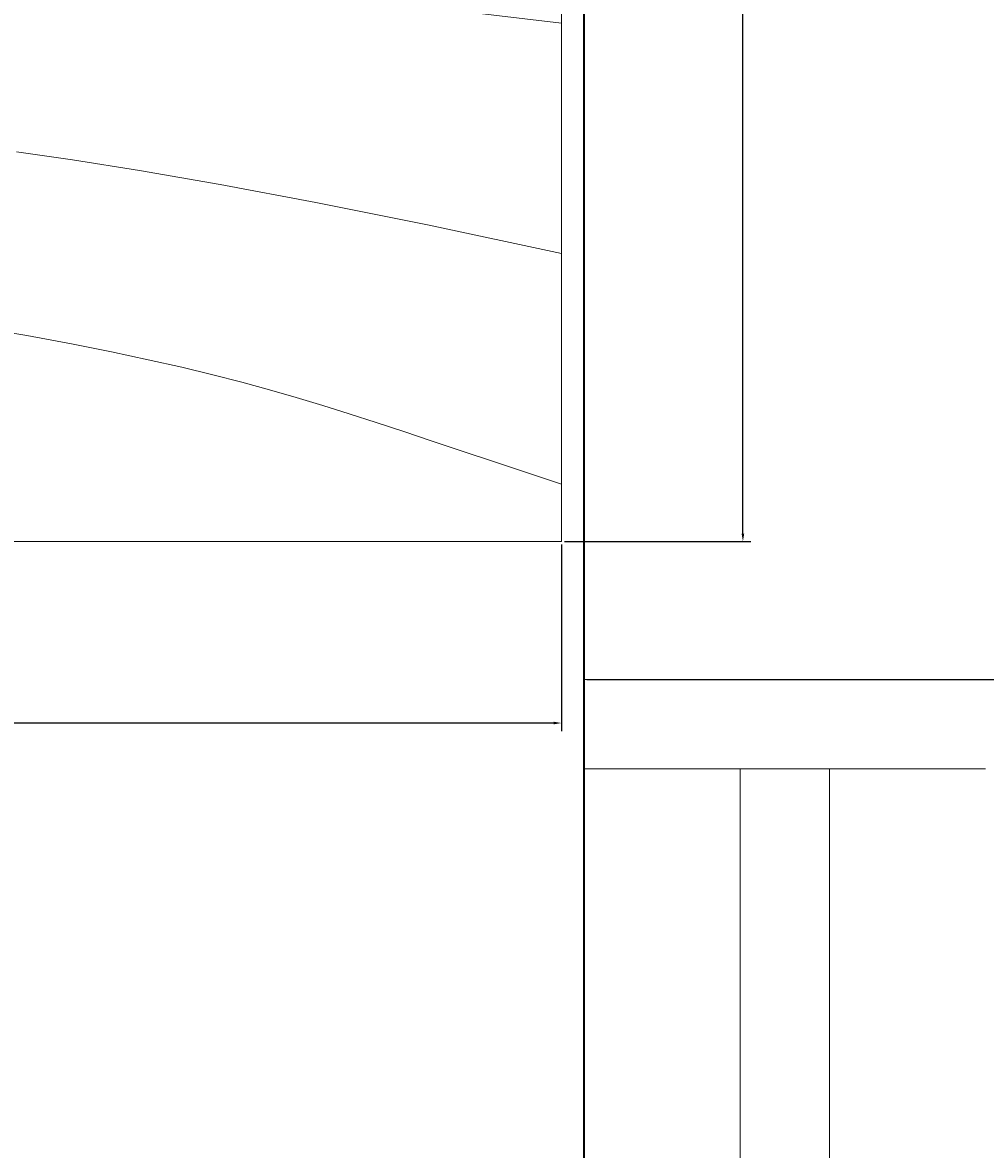
# Model space of a CAD drawing. Units: inches. Extents: x -128 to 854, y -395 to 398.
# Tile 39 of 61: x 292 to 314, y 145 to 170. Entities that reach past the tile are written whole.
import ezdxf

# ---------------------------------------------------------------- set-up
doc = ezdxf.new("R2010")
doc.units = ezdxf.units.IN
doc.header["$MEASUREMENT"] = 0
for name, color, linetype, lineweight in [('A-ANNO-DIMS', 2, 'Continuous', 18), ('A-FURN', 8, 'Continuous', 18), ('A-GLAZ', 220, 'Continuous', 18), ('A-WALL', 4, 'Continuous', 35)]:
    doc.layers.add(name, color=color, linetype=linetype, lineweight=lineweight)
doc.styles.get("Standard").update_dxf_attribs({"font": 'arial.ttf'})
doc.dimstyles.get("Standard").update_dxf_attribs({"dimtxt": 0.18, "dimasz": 0.18, "dimexe": 0.18, "dimexo": 0.0625, "dimgap": 0.09, "dimtad": 0, "dimtih": 1, "dimtoh": 1, "dimdec": 1, "dimzin": 0, "dimdsep": 46, "dimlunit": 4, "dimtxsty": 'Standard', "dimcen": 0.09, "dimclrd": 1, "dimclre": 2, "dimclrt": 6, "dimadec": 0, "dimazin": 0, "dimtfac": 1, "dimtdec": 1, "dimtofl": 0, "dimtmove": 0, "dimatfit": 3, "dimfxl": 1, "dimtfill": 2, "dimtfillclr": 3, "dimtolj": 1, "dimtzin": 0, "dimarcsym": 0})

# ---------------------------------------------------------------- blocks, each defined once
blk = doc.blocks.new('Table - Square Woodgrain 42 x 42 in.')
blk.add_line((0, -42), (42, -42))
for points in [[(0, -42), (0, 0), (42, 0), (42, -42)], [(0, -24), (3.9243, -23.6805), (7.4766, -23.4138), (10.6891, -23.1954), (13.5943, -23.0205), (16.2247, -22.8847), (18.6125, -22.7832), (20.7903, -22.7116), (22.7903, -22.6651), (24.6563, -22.642), (26.4764, -22.6507), (28.35, -22.7024), (30.3766, -22.8084), (32.6555, -22.98), (35.2861, -23.2283), (38.3678, -23.5645), (42, -24)], [(42, -32), (37.392, -31.017), (33.4585, -30.2231), (30.1291, -29.5949), (27.3334, -29.109), (25.0009, -28.742), (23.0612, -28.4707)], [(21.6171, -34.5413), (23.4136, -34.8486), (24.9657, -35.1382), (26.3614, -35.4156), (27.6332, -35.6841), (28.7995, -35.9467), (29.8788, -36.2064), (30.8897, -36.4661), (31.8507, -36.7288), (32.7802, -36.9973), (33.6968, -37.2747), (34.6175, -37.5635), (35.5531, -37.8651), (36.5128, -38.1805), (37.506, -38.5108), (38.5421, -38.8568), (39.6302, -39.2197), (40.7797, -39.6004), (42, -40)]]:
    blk.add_lwpolyline(points)
blk = doc.blocks.new('*D55')
at = {"layer": 'A-ANNO-DIMS', "color": 0, "lineweight": -2, "transparency": 16777216}
for p, q in [((304.81, 186.741), (221.092, 186.741)), ((221.272, 181.741), (221.272, 131.873)), ((221.272, 77.741), (221.272, 127.608)), ((304.81, 72.741), (221.092, 72.741))]:
    blk.add_line(p, q, dxfattribs=at)
at = {"layer": 'A-ANNO-DIMS', "color": 0, "transparency": 16777216}
for points in [[(220.439, 181.741), (222.105, 181.741), (221.272, 186.741)], [(220.439, 77.741), (222.105, 77.741), (221.272, 72.741)]]:
    blk.add_solid(points, dxfattribs=at)
at = {"layer": 'Defpoints', "color": 0, "transparency": 16777216}
for p in [(221.272, 186.741), (304.873, 186.741), (304.873, 72.741)]:
    blk.add_point(p, dxfattribs=at)
at = {"layer": 'A-ANNO-DIMS', "color": 0, "transparency": 16777216, "insert": (221.272, 129.741), "char_height": 4, "attachment_point": 5, "bg_fill": 1, "box_fill_scale": 1.25, "bg_fill_color": 3, "bg_fill_transparency": 0}
blk.add_mtext('\\A1;9\'-6"', dxfattribs=at)
blk = doc.blocks.new('WIN-48IN')
for p, q in [((9, 52), (0, 52)), ((9, 50), (0, 50)), ((3.5, 50), (3.5, 2)), ((5.5, 50), (5.5, 2))]:
    blk.add_line(p, q)
blk = doc.blocks.new('*D87')
at = {"layer": 'A-ANNO-DIMS', "color": 2, "lineweight": -2, "transparency": 16777216}
for p, q in [((304.435, 185.918), (308.616, 185.918)), ((304.435, 158.828), (308.616, 158.828))]:
    blk.add_line(p, q, dxfattribs=at)
at = {"layer": 'A-ANNO-DIMS', "color": 1, "lineweight": -2, "transparency": 16777216}
for p, q in [((308.436, 185.738), (308.436, 172.557)), ((308.436, 159.008), (308.436, 172.19))]:
    blk.add_line(p, q, dxfattribs=at)
at = {"layer": 'A-ANNO-DIMS', "color": 1, "transparency": 16777216}
for points in [[(308.406, 185.738), (308.466, 185.738), (308.436, 185.918)], [(308.406, 159.008), (308.466, 159.008), (308.436, 158.828)]]:
    blk.add_solid(points, dxfattribs=at)
at = {"layer": 'Defpoints', "color": 0, "transparency": 16777216}
for p in [(304.372, 185.918), (308.436, 185.918), (304.372, 158.828)]:
    blk.add_point(p, dxfattribs=at)
at = {"layer": 'A-ANNO-DIMS', "color": 6, "transparency": 16777216, "insert": (308.436, 172.373), "char_height": 0.18, "attachment_point": 5, "bg_fill": 1, "box_fill_scale": 1.25, "bg_fill_color": 3, "bg_fill_transparency": 0}
blk.add_mtext('\\A1;SIDE TABLE 2\'-3" TYP.', dxfattribs=at)
blk = doc.blocks.new('*D88')
at = {"layer": 'A-ANNO-DIMS', "color": 2, "lineweight": -2, "transparency": 16777216}
for p, q in [((277.284, 158.766), (277.284, 154.585)), ((304.372, 158.766), (304.372, 154.585))]:
    blk.add_line(p, q, dxfattribs=at)
at = {"layer": 'A-ANNO-DIMS', "color": 1, "lineweight": -2, "transparency": 16777216}
for p, q in [((277.464, 154.765), (290.188, 154.765)), ((304.192, 154.765), (291.468, 154.765))]:
    blk.add_line(p, q, dxfattribs=at)
at = {"layer": 'A-ANNO-DIMS', "color": 1, "transparency": 16777216}
for points in [[(277.464, 154.795), (277.464, 154.735), (277.284, 154.765)], [(304.192, 154.795), (304.192, 154.735), (304.372, 154.765)]]:
    blk.add_solid(points, dxfattribs=at)
at = {"layer": 'Defpoints', "color": 0, "transparency": 16777216}
for p in [(277.284, 158.828), (304.372, 158.828), (304.372, 154.765)]:
    blk.add_point(p, dxfattribs=at)
at = {"layer": 'A-ANNO-DIMS', "color": 6, "transparency": 16777216, "insert": (290.828, 154.765), "char_height": 0.18, "attachment_point": 5, "bg_fill": 1, "box_fill_scale": 1.25, "bg_fill_color": 3, "bg_fill_transparency": 0}
blk.add_mtext('\\A1;2\'-3" TYP.', dxfattribs=at)
blk = doc.blocks.new('*D98')
at = {"layer": 'A-ANNO-DIMS', "color": 2, "lineweight": -2, "transparency": 16777216}
for p, q in [((313.935, 348.741), (351.853, 348.741)), ((313.935, -89.259), (351.853, -89.259))]:
    blk.add_line(p, q, dxfattribs=at)
at = {"layer": 'A-ANNO-DIMS', "color": 1, "lineweight": -2, "transparency": 16777216}
for p, q in [((351.673, 348.561), (351.673, 129.923)), ((351.673, -89.079), (351.673, 129.559))]:
    blk.add_line(p, q, dxfattribs=at)
at = {"layer": 'A-ANNO-DIMS', "color": 1, "transparency": 16777216}
for points in [[(351.643, 348.561), (351.703, 348.561), (351.673, 348.741)], [(351.643, -89.079), (351.703, -89.079), (351.673, -89.259)]]:
    blk.add_solid(points, dxfattribs=at)
at = {"layer": 'Defpoints', "color": 0, "transparency": 16777216}
for p in [(313.873, 348.741), (351.673, 348.741), (313.873, -89.259)]:
    blk.add_point(p, dxfattribs=at)
at = {"layer": 'A-ANNO-DIMS', "color": 6, "transparency": 16777216, "insert": (351.673, 129.741), "char_height": 0.18, "attachment_point": 5, "bg_fill": 1, "box_fill_scale": 1.25, "bg_fill_color": 3, "bg_fill_transparency": 0}
blk.add_mtext('\\A1;36\'-6"', dxfattribs=at)
blk = doc.blocks.new('*D112')
at = {"layer": 'A-ANNO-DIMS', "color": 2, "lineweight": -2, "transparency": 16777216}
for p, q in [((304.935, 186.741), (351.853, 186.741)), ((304.935, 155.741), (351.853, 155.741))]:
    blk.add_line(p, q, dxfattribs=at)
at = {"layer": 'A-ANNO-DIMS', "color": 1, "lineweight": -2, "transparency": 16777216}
for p, q in [((351.673, 186.561), (351.673, 171.421)), ((351.673, 155.921), (351.673, 171.06))]:
    blk.add_line(p, q, dxfattribs=at)
at = {"layer": 'A-ANNO-DIMS', "color": 1, "transparency": 16777216}
for points in [[(351.643, 186.561), (351.703, 186.561), (351.673, 186.741)], [(351.643, 155.921), (351.703, 155.921), (351.673, 155.741)]]:
    blk.add_solid(points, dxfattribs=at)
at = {"layer": 'Defpoints', "color": 0, "transparency": 16777216}
for p in [(304.873, 186.741), (304.873, 155.741), (351.673, 155.741)]:
    blk.add_point(p, dxfattribs=at)
at = {"layer": 'A-ANNO-DIMS', "color": 6, "transparency": 16777216, "insert": (351.673, 171.241), "char_height": 0.18, "attachment_point": 5, "bg_fill": 1, "box_fill_scale": 1.25, "bg_fill_color": 3, "bg_fill_transparency": 0}
blk.add_mtext('\\A1;2\'-7"', dxfattribs=at)

msp = doc.modelspace()

# ---------------------------------------------------------------- linework, layer by layer
at = {"layer": 'A-WALL'}
msp.add_line((304.873, 186.741), (304.873, 72.741), dxfattribs=at)

# ---------------------------------------------------------------- block references
at = {"layer": 'A-FURN', "xscale": 0.6449685946951323, "yscale": 0.6449685946951323, "zscale": 0.6449685946951323}
msp.add_blockref('Table - Square Woodgrain 42 x 42 in.', (277.284, 185.917), dxfattribs=at)
at = {"layer": 'A-GLAZ', "extrusion": (0, 0, -1), "zscale": -1}
msp.add_blockref('WIN-48IN', (-313.873, 103.741), dxfattribs=at)

# ---------------------------------------------------------------- dimensions: what is measured, and where the dimension line sits
at = {"layer": 'A-ANNO-DIMS'}
for base, p1, p2, override, picture, middle in [((351.673, 348.741), (313.873, -89.259), (313.873, 348.741), {"dimdec": 1, "dimlfac": 1, "dimrnd": 0, "dimzin": 1, "dimdsep": 46, "dimlunit": 4, "dimfrac": 2}, '*D98', (351.673, 129.741)), ((221.272, 186.741), (304.873, 72.741), (304.873, 186.741), {"dimtxt": 4, "dimasz": 5, "dimclrd": 0, "dimclre": 0, "dimclrt": 0}, '*D55', (221.272, 129.741)), ((351.673, 155.741), (304.873, 186.741), (304.873, 155.741), {"dimdec": 1, "dimlfac": 1, "dimrnd": 0, "dimzin": 1, "dimdsep": 46, "dimlunit": 4, "dimfrac": 2}, '*D112', (351.673, 171.241))]:
    dim = msp.add_linear_dim(base=base, p1=p1, p2=p2, angle=90, dimstyle='Standard', override=override, dxfattribs=at)
    dim.commit()
    dim.dimension.update_dxf_attribs({"geometry": picture, "text_midpoint": middle})
dim = msp.add_linear_dim(base=(308.436, 185.918), p1=(304.372, 158.828), p2=(304.372, 185.918), angle=90, text='SIDE TABLE <> TYP.', dimstyle='Standard', override={"dimdec": 1, "dimlfac": 1, "dimrnd": 0, "dimzin": 1, "dimdsep": 46, "dimlunit": 4, "dimfrac": 2}, dxfattribs=at)
dim.commit()
dim.dimension.update_dxf_attribs({"geometry": '*D87', "text_midpoint": (308.436, 172.373)})
dim = msp.add_linear_dim(base=(304.372, 154.765), p1=(277.284, 158.828), p2=(304.372, 158.828), text='<> TYP.', dimstyle='Standard', override={"dimdec": 1, "dimlfac": 1, "dimrnd": 0, "dimzin": 1, "dimdsep": 46, "dimlunit": 4, "dimfrac": 2}, dxfattribs=at)
dim.commit()
dim.dimension.update_dxf_attribs({"geometry": '*D88', "text_midpoint": (290.828, 154.765)})

doc.saveas('drawing.dxf')
